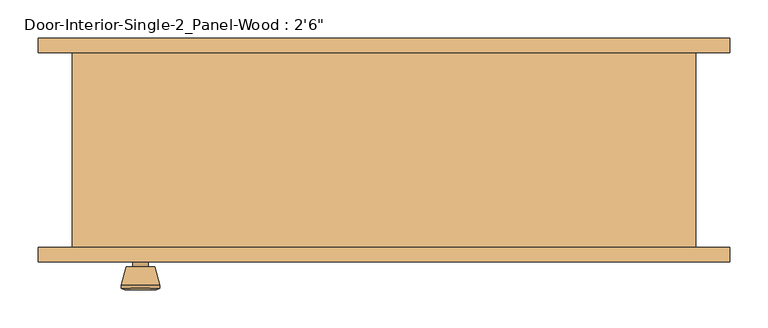
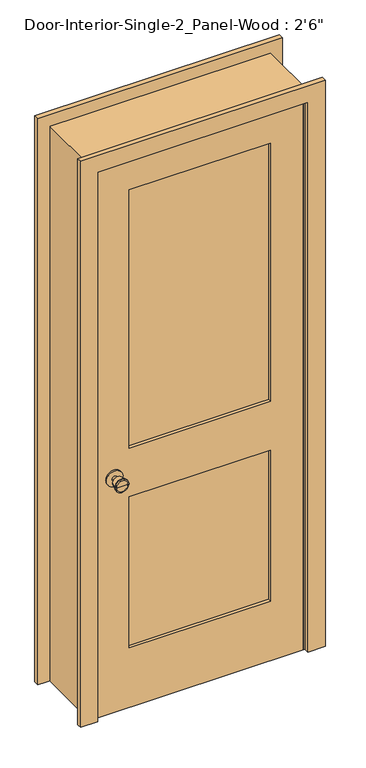
"""IFC4 building model written with IfcOpenShell, lengths in millimetres: door geometry."""

from ifc_helpers import new_model, si_unit, point, frame, frame_2d, origin, place, context, project, spatial, polyline, circle_curve, trimmed, segment, composite_curve, outline, extrude, faceted_brep, source, transform, mapped, element, save
from ifc_brep_helpers import plane_surface, cylinder_surface, revolved_surface, advanced_brep


def door_e3d10b2c(model_context):
    return source(origin(), model_context, "Body", "SolidModel", [
        advanced_brep(
        [(-317.5, -82.9, 914.4), (-327.5, -82.9, 914.4), (-307.5, -82.9, 914.4), (-297.0241324, -33.9, 914.4), (-337.9758676, -33.9, 914.4), (-317.5, -33.9, 914.4), (-292.5, -35.7278681, 914.4), (-342.5, -35.7278681, 914.4), (-292.5, -39.1915463, 914.4), (-342.5, -39.1915463, 914.4), (-298.863764, -63.9, 914.4), (-336.136236, -63.9, 914.4), (-307.5, -63.9, 914.4), (-327.5, -63.9, 914.4)],
        [
            (0, 1),
            (1, 2, circle_curve(frame((-317.5, -82.9, 914.4), z_axis=(0.0, -1.0, 0.0), x_axis=(-1.0, 0.0, 0.0)), 10.0)),
            (2, 0),
            (2, 1, circle_curve(frame((-317.5, -82.9, 914.4), z_axis=(0.0, -1.0, 0.0), x_axis=(-1.0, 0.0, 0.0)), 10.0)),
            (3, 4, circle_curve(frame((-317.5, -33.9, 914.4), z_axis=(0.0, 1.0, 0.0), x_axis=(-1.0, 0.0, 0.0)), 20.4758676)),
            (4, 5),
            (5, 3),
            (4, 3, circle_curve(frame((-317.5, -33.9, 914.4), z_axis=(0.0, 1.0, 0.0), x_axis=(-1.0, 0.0, 0.0)), 20.4758676)),
            (6, 7, circle_curve(frame((-317.5, -35.7278681, 914.4), z_axis=(0.0, 1.0, 0.0), x_axis=(-1.0, 0.0, 0.0)), 25.0)),
            (7, 4),
            (3, 6),
            (7, 6, circle_curve(frame((-317.5, -35.7278681, 914.4), z_axis=(0.0, 1.0, 0.0), x_axis=(-1.0, 0.0, 0.0)), 25.0)),
            (8, 9, circle_curve(frame((-317.5, -39.1915463, 914.4), z_axis=(0.0, 1.0, 0.0), x_axis=(-1.0, 0.0, 0.0)), 25.0)),
            (9, 7),
            (6, 8),
            (9, 8, circle_curve(frame((-317.5, -39.1915463, 914.4), z_axis=(0.0, 1.0, 0.0), x_axis=(-1.0, 0.0, 0.0)), 25.0)),
            (10, 11, circle_curve(frame((-317.5, -63.9, 914.4), z_axis=(0.0, 1.0, 0.0), x_axis=(-1.0, 0.0, 0.0)), 18.636236)),
            (11, 9),
            (8, 10),
            (11, 10, circle_curve(frame((-317.5, -63.9, 914.4), z_axis=(0.0, 1.0, 0.0), x_axis=(-1.0, 0.0, 0.0)), 18.636236)),
            (12, 13, circle_curve(frame((-317.5, -63.9, 914.4), z_axis=(0.0, 1.0, 0.0), x_axis=(-1.0, 0.0, 0.0)), 10.0)),
            (13, 11),
            (10, 12),
            (13, 12, circle_curve(frame((-317.5, -63.9, 914.4), z_axis=(0.0, 1.0, 0.0), x_axis=(-1.0, 0.0, 0.0)), 10.0)),
            (1, 13),
            (12, 2),
        ],
        [
            plane_surface(frame((-317.5, -82.9, 914.4), z_axis=(0.0, -1.0, 0.0), x_axis=(-1.0, 0.0, 0.0))),
            plane_surface(frame((-317.5, -33.9, 914.4), z_axis=(0.0, 1.0, 0.0), x_axis=(-1.0, 0.0, 0.0))),
            revolved_surface(polyline([(-337.9758676, -33.9, 914.4), (-342.5, -35.7278681, 914.4)]), (-317.5, -82.9, 914.4), (0.0, -1.0, 0.0)),
            cylinder_surface(frame((-317.5, -82.9, 914.4), z_axis=(0.0, -1.0, 0.0), x_axis=(-1.0, 0.0, 0.0)), 25.0),
            revolved_surface(polyline([(-342.5, -39.1915463, 914.4), (-336.136236, -63.9, 914.4)]), (-317.5, -82.9, 914.4), (0.0, -1.0, 0.0)),
            plane_surface(frame((-317.5, -63.9, 914.4), z_axis=(0.0, -1.0, 0.0), x_axis=(-1.0, 0.0, 0.0))),
            cylinder_surface(frame((-317.5, -82.9, 914.4), z_axis=(0.0, -1.0, 0.0), x_axis=(-1.0, 0.0, 0.0)), 10.0),
        ],
        [
            (0, [[1, 2, 3]]),
            (0, [[-3, 4, -1]]),
            (1, [[5, 6, 7]]),
            (1, [[8, -7, -6]]),
            (2, [[9, 10, -5, 11]]),
            (2, [[12, -11, -8, -10]]),
            (3, [[13, 14, -9, 15]]),
            (3, [[16, -15, -12, -14]]),
            (4, [[17, 18, -13, 19]]),
            (4, [[20, -19, -16, -18]]),
            (5, [[21, 22, -17, 23]]),
            (5, [[24, -23, -20, -22]]),
            (6, [[-2, 25, -21, 26]]),
            (6, [[-4, -26, -24, -25]]),
        ],
    ),
        extrude(outline(composite_curve([segment(trimmed(circle_curve(frame_2d((914.4, -317.5)), 30.0), [point((914.4, -347.5))], [point((914.4, -287.5))], False, "CARTESIAN"), True, "CONTINUOUS"), segment(trimmed(circle_curve(frame_2d((914.4, -317.5)), 30.0), [point((914.4, -287.5))], [point((914.4, -347.5))], False, "CARTESIAN"), True, "CONTINUOUS")], self_intersect=False)), frame((0.0, -88.9, 0.0), z_axis=(0.0, 1.0, 0.0), x_axis=(0.0, 0.0, 1.0)), (0.0, 0.0, 1.0), 6.0),
        advanced_brep(
        [(-317.5, -129.825, 914.4), (-307.5, -129.825, 914.4), (-327.5, -129.825, 914.4), (-297.0241324, -178.825, 914.4), (-317.5, -178.825, 914.4), (-337.9758676, -178.825, 914.4), (-292.5, -176.9971319, 914.4), (-342.5, -176.9971319, 914.4), (-292.5, -173.5334537, 914.4), (-342.5, -173.5334537, 914.4), (-298.863764, -148.825, 914.4), (-336.136236, -148.825, 914.4), (-307.5, -148.825, 914.4), (-327.5, -148.825, 914.4)],
        [
            (0, 1),
            (1, 2, circle_curve(frame((-317.5, -129.825, 914.4), z_axis=(0.0, 1.0, 0.0), x_axis=(-1.0, 0.0, 0.0)), 10.0)),
            (2, 0),
            (2, 1, circle_curve(frame((-317.5, -129.825, 914.4), z_axis=(0.0, 1.0, 0.0), x_axis=(-1.0, 0.0, 0.0)), 10.0)),
            (3, 4),
            (4, 5),
            (5, 3, circle_curve(frame((-317.5, -178.825, 914.4), z_axis=(0.0, -1.0, 0.0), x_axis=(-1.0, 0.0, 0.0)), 20.4758676)),
            (3, 5, circle_curve(frame((-317.5, -178.825, 914.4), z_axis=(0.0, -1.0, 0.0), x_axis=(-1.0, 0.0, 0.0)), 20.4758676)),
            (6, 3),
            (5, 7),
            (7, 6, circle_curve(frame((-317.5, -176.9971319, 914.4), z_axis=(0.0, -1.0, 0.0), x_axis=(-1.0, 0.0, 0.0)), 25.0)),
            (6, 7, circle_curve(frame((-317.5, -176.9971319, 914.4), z_axis=(0.0, -1.0, 0.0), x_axis=(-1.0, 0.0, 0.0)), 25.0)),
            (8, 6),
            (7, 9),
            (9, 8, circle_curve(frame((-317.5, -173.5334537, 914.4), z_axis=(0.0, -1.0, 0.0), x_axis=(-1.0, 0.0, 0.0)), 25.0)),
            (8, 9, circle_curve(frame((-317.5, -173.5334537, 914.4), z_axis=(0.0, -1.0, 0.0), x_axis=(-1.0, 0.0, 0.0)), 25.0)),
            (10, 8),
            (9, 11),
            (11, 10, circle_curve(frame((-317.5, -148.825, 914.4), z_axis=(0.0, -1.0, 0.0), x_axis=(-1.0, 0.0, 0.0)), 18.636236)),
            (10, 11, circle_curve(frame((-317.5, -148.825, 914.4), z_axis=(0.0, -1.0, 0.0), x_axis=(-1.0, 0.0, 0.0)), 18.636236)),
            (12, 10),
            (11, 13),
            (13, 12, circle_curve(frame((-317.5, -148.825, 914.4), z_axis=(0.0, -1.0, 0.0), x_axis=(-1.0, 0.0, 0.0)), 10.0)),
            (12, 13, circle_curve(frame((-317.5, -148.825, 914.4), z_axis=(0.0, -1.0, 0.0), x_axis=(-1.0, 0.0, 0.0)), 10.0)),
            (1, 12),
            (13, 2),
        ],
        [
            plane_surface(frame((-317.5, -129.825, 914.4), z_axis=(0.0, 1.0, 0.0), x_axis=(-1.0, 0.0, 0.0))),
            plane_surface(frame((-317.5, -178.825, 914.4), z_axis=(0.0, -1.0, 0.0), x_axis=(-1.0, 0.0, 0.0))),
            revolved_surface(polyline([(-337.9758676, -178.825, 914.4), (-342.5, -176.9971319, 914.4)]), (-317.5, -129.825, 914.4), (0.0, 1.0, 0.0)),
            cylinder_surface(frame((-317.5, -129.825, 914.4), z_axis=(0.0, 1.0, 0.0), x_axis=(-1.0, 0.0, 0.0)), 25.0),
            revolved_surface(polyline([(-342.5, -173.5334537, 914.4), (-336.136236, -148.825, 914.4)]), (-317.5, -129.825, 914.4), (0.0, 1.0, 0.0)),
            plane_surface(frame((-317.5, -148.825, 914.4), z_axis=(0.0, 1.0, 0.0), x_axis=(-1.0, 0.0, 0.0))),
            cylinder_surface(frame((-317.5, -129.825, 914.4), z_axis=(0.0, 1.0, 0.0), x_axis=(-1.0, 0.0, 0.0)), 10.0),
        ],
        [
            (0, [[1, 2, 3]]),
            (0, [[-3, 4, -1]]),
            (1, [[5, 6, 7]]),
            (1, [[-6, -5, 8]]),
            (2, [[9, -7, 10, 11]]),
            (2, [[-10, -8, -9, 12]]),
            (3, [[13, -11, 14, 15]]),
            (3, [[-14, -12, -13, 16]]),
            (4, [[17, -15, 18, 19]]),
            (4, [[-18, -16, -17, 20]]),
            (5, [[21, -19, 22, 23]]),
            (5, [[-22, -20, -21, 24]]),
            (6, [[25, -23, 26, -2]]),
            (6, [[-26, -24, -25, -4]]),
        ],
    ),
        extrude(outline(composite_curve([segment(trimmed(circle_curve(frame_2d((914.4, -317.5)), 30.0), [point((914.4, -347.5))], [point((914.4, -287.5))], False, "CARTESIAN"), True, "CONTINUOUS"), segment(trimmed(circle_curve(frame_2d((914.4, -317.5)), 30.0), [point((914.4, -287.5))], [point((914.4, -347.5))], False, "CARTESIAN"), True, "CONTINUOUS")], self_intersect=False)), frame((0.0, -129.825, 0.0), z_axis=(0.0, 1.0, 0.0), x_axis=(0.0, 0.0, 1.0)), (0.0, 0.0, 1.0), 6.0),
        faceted_brep([(406.4, -123.825, 0.0), (381.0, -123.825, 0.0), (381.0, -88.9, 0.0), (368.3, -88.9, 0.0), (368.3, -53.975, 0.0), (381.0, -53.975, 0.0), (381.0, 130.175, 0.0), (406.4, 130.175, 0.0), (406.4, 130.175, 2159.0), (406.4, -123.825, 2159.0), (381.0, 130.175, 2133.6), (-381.0, 130.175, 2133.6), (-381.0, 130.175, 0.0), (-406.4, 130.175, 0.0), (-406.4, 130.175, 2159.0), (381.0, -53.975, 2133.6), (368.3, -53.975, 2120.9), (-368.3, -53.975, 2120.9), (-368.3, -53.975, 0.0), (-381.0, -53.975, 0.0), (-381.0, -53.975, 2133.6), (368.3, -88.9, 2120.9), (381.0, -88.9, 2133.6), (-381.0, -88.9, 2133.6), (-381.0, -88.9, 0.0), (-368.3, -88.9, 0.0), (-368.3, -88.9, 2120.9), (381.0, -123.825, 2133.6), (-406.4, -123.825, 2159.0), (-406.4, -123.825, 0.0), (-381.0, -123.825, 0.0), (-381.0, -123.825, 2133.6)], [[[0, 1, 2, 3, 4, 5, 6, 7]], [[7, 8, 9, 0]], [[6, 10, 11, 12, 13, 14, 8, 7]], [[5, 15, 10, 6]], [[4, 16, 17, 18, 19, 20, 15, 5]], [[3, 21, 16, 4]], [[2, 22, 23, 24, 25, 26, 21, 3]], [[1, 27, 22, 2]], [[0, 9, 28, 29, 30, 31, 27, 1]], [[8, 14, 28, 9]], [[15, 20, 11, 10]], [[21, 26, 17, 16]], [[27, 31, 23, 22]], [[29, 13, 12, 19, 18, 25, 24, 30]], [[14, 13, 29, 28]], [[20, 19, 12, 11]], [[26, 25, 18, 17]], [[31, 30, 24, 23]]]),
        extrude(outline(polyline([(2133.6, -381.0), (0.0, -381.0), (0.0, 381.0), (2133.6, 381.0), (2133.6, -381.0)]), holes=[polyline([(2014.5375, -260.35), (2014.5375, 260.35), (1009.65, 260.35), (1009.65, -260.35), (2014.5375, -260.35)]), polyline([(819.15, -260.35), (819.15, 260.35), (231.775, 260.35), (231.775, -260.35), (819.15, -260.35)])]), frame((0.0, -123.825, 0.0), z_axis=(0.0, 1.0, 0.0), x_axis=(0.0, 0.0, 1.0)), (0.0, 0.0, 1.0), 34.925),
        extrude(outline(polyline([(260.35, -100.5416667), (260.35, -112.1833333), (-260.35, -112.1833333), (-260.35, -100.5416667), (260.35, -100.5416667)])), frame((0.0, 0.0, 1009.65), z_axis=(0.0, 0.0, 1.0), x_axis=(1.0, 0.0, 0.0)), (0.0, 0.0, 1.0), 1004.8875),
        extrude(outline(polyline([(260.35, -100.5416667), (260.35, -112.1833333), (-260.35, -112.1833333), (-260.35, -100.5416667), (260.35, -100.5416667)])), frame((0.0, 0.0, 231.775), z_axis=(0.0, 0.0, 1.0), x_axis=(1.0, 0.0, 0.0)), (0.0, 0.0, 1.0), 587.375),
        extrude(outline(polyline([(0.0, 450.85), (2203.45, 450.85), (2203.45, -450.85), (0.0, -450.85), (0.0, -387.35), (2139.95, -387.35), (2139.95, 387.35), (0.0, 387.35), (0.0, 450.85)])), frame((0.0, -142.875, 0.0), z_axis=(0.0, 1.0, 0.0), x_axis=(0.0, 0.0, 1.0)), (0.0, 0.0, 1.0), 19.05),
        extrude(outline(polyline([(0.0, 450.85), (2203.45, 450.85), (2203.45, -450.85), (0.0, -450.85), (0.0, -387.35), (2139.95, -387.35), (2139.95, 387.35), (0.0, 387.35), (0.0, 450.85)])), frame((0.0, 130.175, 0.0), z_axis=(0.0, 1.0, 0.0), x_axis=(0.0, 0.0, 1.0)), (0.0, 0.0, 1.0), 19.05),
    ])


if __name__ == "__main__":
    model = new_model("IFC4")
    model_context = context("Model", 3, world=origin())
    ifc_project = project(units=[si_unit("LENGTHUNIT", "METRE", prefix="MILLI")], contexts=[model_context])
    site = spatial("IfcSite", under=ifc_project)
    building = spatial("IfcBuilding", under=site)
    placement = place(None, origin())
    door_shape = door_e3d10b2c(model_context)
    element("IfcDoor", 1, ObjectType="Door-Interior-Single-2_Panel-Wood : 2'6\"", at=placement, inside=building, context=model_context, shape_type="MappedRepresentation", body=[
        mapped(door_shape, transform((0.0, 0.0, 0.0), x_axis=(1.0, 0.0, 0.0), y_axis=(0.0, 1.0, 0.0), z_axis=(0.0, 0.0, 1.0))),
    ])
    save(model, "model.ifc")

# Revit data of these elements
# Type "Door-Interior-Single-2_Panel-Wood : 2'6\""
#   Type Mark = "10"
#   Assembly Code = "C1020300"
#   Analytic Construction = "Wooden"
#   Top Rail = 0' - 4 11/16"
#   Thickness = 0' - 1 3/8"
#   Thermal Resistance (R) = 2.5876 (h·ft²·°F)/BTU
#   Swing Angle [instance default] = 90.00°
#   Stiles = 0' - 4 3/4"
#   Rough Width = 2' - 8"
#   Rough Height = 7' - 1"
#   Lock Rail = 0' - 7 1/2"
#   Height = 7' - 0"
#   Width = 2' - 6"
#   Heat Transfer Coefficient (U) = 0.3865 BTU/(h·ft²·°F)
#   Bottom Rail = 0' - 9 1/8"
#   Trim Material = Cherry
#   Panel Material = Cherry
#   Frame Material = Cherry
#   Door Handle Material = Aluminum
#   Visual Light Transmittance = 0
#   Solar Heat Gain Coefficient = 0
#   Wall Closure = (empty or 0)
#   Function = (empty or 0)
# Element 1 (IfcDoor, "Door-Interior-Single-2_Panel-Wood : 2'6\"")
#   Materials on its faces: "Cherry", "Aluminum"
# Materials
#   "Cherry": class "Wood", colour RGB 226 177 128, transparency 0, Description = "Prunus Serotina", Cost = 0
#   "Aluminum": class "Metal", colour RGB 247 247 247, transparency 0, Description = "Aluminum 6061", Cost = 0
